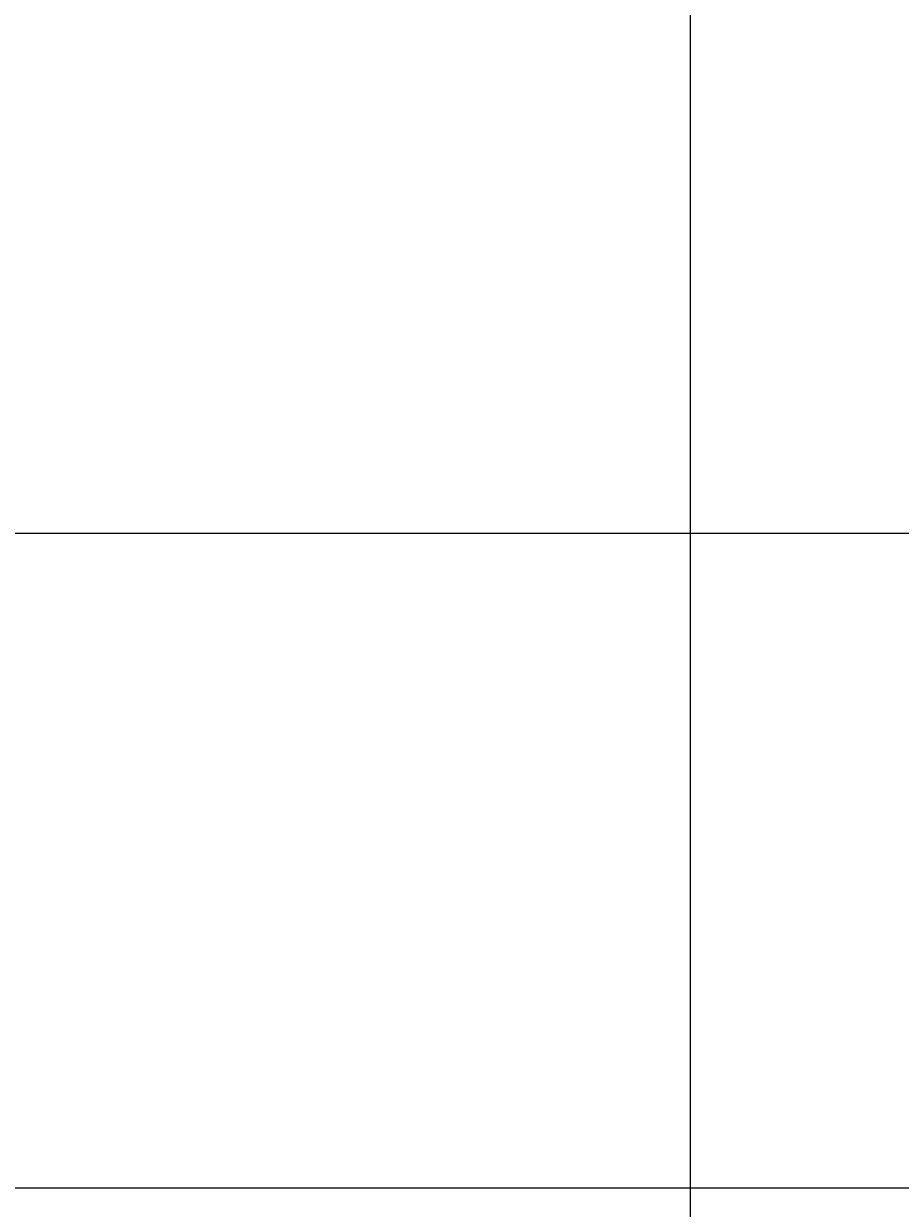
# Model space of a CAD drawing. Units: inches. Extents: x 35362 to 73946, y 43607 to 67532.
# Tile 76 of 134: x 49302 to 50119, y 47689 to 48793. Entities that reach past the tile are written whole.
import ezdxf

# ---------------------------------------------------------------- set-up
doc = ezdxf.new("R2010")
doc.units = ezdxf.units.IN
doc.header["$MEASUREMENT"] = 0
doc.layers.add('A-ANNO-DIMS', color=2, linetype='Continuous', lineweight=18)
doc.styles.get("Standard").update_dxf_attribs({"font": 'arial.ttf'})
doc.dimstyles.get("Standard").update_dxf_attribs({"dimtxt": 0.18, "dimasz": 0.18, "dimexe": 0.18, "dimexo": 0.0625, "dimgap": 0.09, "dimtad": 0, "dimtih": 1, "dimtoh": 1, "dimdec": 4, "dimzin": 0, "dimdsep": 46, "dimtxsty": 'Standard', "dimcen": 0.09, "dimadec": 0, "dimazin": 0, "dimtfac": 1, "dimtdec": 4, "dimtofl": 0, "dimtmove": 0, "dimatfit": 3, "dimfxl": 1, "dimtolj": 1, "dimtzin": 0, "dimarcsym": 0})

# ---------------------------------------------------------------- blocks, each defined once
blk = doc.blocks.new('*D11')
at = {"layer": 'A-ANNO-DIMS', "color": 0, "lineweight": -2, "transparency": 16777216}
for p, q in [((47978.7, 56028.8), (47978.7, 43606.7)), ((53109.8, 56028.8), (53109.8, 43606.7)), ((47978.8, 43606.9), (50543.9, 43606.9)), ((53109.6, 43606.9), (50544.6, 43606.9))]:
    blk.add_line(p, q, dxfattribs=at)
at = {"layer": 'A-ANNO-DIMS', "color": 0, "transparency": 16777216}
for points in [[(47978.8, 43606.9), (47978.8, 43606.8), (47978.7, 43606.9)], [(53109.6, 43606.9), (53109.6, 43606.8), (53109.8, 43606.9)]]:
    blk.add_solid(points, dxfattribs=at)
at = {"layer": 'Defpoints', "color": 0, "transparency": 16777216}
for p in [(47978.7, 56028.8), (53109.8, 56028.8), (53109.8, 43606.9)]:
    blk.add_point(p, dxfattribs=at)
at = {"layer": 'A-ANNO-DIMS', "color": 0, "transparency": 16777216, "insert": (50544.2, 43606.9), "char_height": 0.18, "attachment_point": 5}
blk.add_mtext('\\A1;5131', dxfattribs=at)
blk = doc.blocks.new('*D13')
at = {"layer": 'A-ANNO-DIMS', "color": 0, "lineweight": -2, "transparency": 16777216}
for p, q in [((48373.5, 51694), (48373.5, 43606.7)), ((51029, 51694), (51029, 43606.7)), ((48373.7, 43606.9), (49700.8, 43606.9)), ((51028.9, 43606.9), (49701.7, 43606.9))]:
    blk.add_line(p, q, dxfattribs=at)
at = {"layer": 'A-ANNO-DIMS', "color": 0, "transparency": 16777216}
for points in [[(48373.7, 43606.9), (48373.7, 43606.8), (48373.5, 43606.9)], [(51028.9, 43606.9), (51028.9, 43606.8), (51029, 43606.9)]]:
    blk.add_solid(points, dxfattribs=at)
at = {"layer": 'Defpoints', "color": 0, "transparency": 16777216}
for p in [(48373.5, 51694.1), (51029, 51694.1), (51029, 43606.9)]:
    blk.add_point(p, dxfattribs=at)
at = {"layer": 'A-ANNO-DIMS', "color": 0, "transparency": 16777216, "insert": (49701.3, 43606.9), "char_height": 0.18, "attachment_point": 5}
blk.add_mtext('\\A1;2655.6', dxfattribs=at)
blk = doc.blocks.new('*D17')
at = {"layer": 'A-ANNO-DIMS', "color": 0, "lineweight": -2, "transparency": 16777216}
for p, q in [((49923.3, 61293.2), (49923.3, 43606.7)), ((51913.9, 61293.2), (51913.9, 43606.7)), ((49923.5, 43606.9), (50918.2, 43606.9)), ((51913.8, 43606.9), (50919.1, 43606.9))]:
    blk.add_line(p, q, dxfattribs=at)
at = {"layer": 'A-ANNO-DIMS', "color": 0, "transparency": 16777216}
for points in [[(49923.5, 43606.9), (49923.5, 43606.8), (49923.3, 43606.9)], [(51913.8, 43606.9), (51913.8, 43606.8), (51913.9, 43606.9)]]:
    blk.add_solid(points, dxfattribs=at)
at = {"layer": 'Defpoints', "color": 0, "transparency": 16777216}
for p in [(49923.3, 61293.3), (51913.9, 61293.3), (51913.9, 43606.9)]:
    blk.add_point(p, dxfattribs=at)
at = {"layer": 'A-ANNO-DIMS', "color": 0, "transparency": 16777216, "insert": (50918.6, 43606.9), "char_height": 0.18, "attachment_point": 5}
blk.add_mtext('\\A1;1990.6', dxfattribs=at)
blk = doc.blocks.new('*D67')
at = {"layer": 'A-ANNO-DIMS', "color": 0, "lineweight": -2, "transparency": 16777216}
for p, q in [((56873.5, 53351.5), (35361.8, 53351.5)), ((35361.9, 53351.3), (35361.9, 49400.9)), ((35361.9, 45450.1), (35361.9, 49400.5)), ((53793.6, 45449.9), (35361.8, 45449.9))]:
    blk.add_line(p, q, dxfattribs=at)
at = {"layer": 'A-ANNO-DIMS', "color": 0, "transparency": 16777216}
for points in [[(35361.9, 53351.3), (35362, 53351.3), (35361.9, 53351.5)], [(35361.9, 45450.1), (35362, 45450.1), (35361.9, 45449.9)]]:
    blk.add_solid(points, dxfattribs=at)
at = {"layer": 'Defpoints', "color": 0, "transparency": 16777216}
for p in [(35361.9, 53351.5), (56873.6, 53351.5), (53793.6, 45449.9)]:
    blk.add_point(p, dxfattribs=at)
at = {"layer": 'A-ANNO-DIMS', "color": 0, "transparency": 16777216, "insert": (35361.9, 49400.7), "char_height": 0.18, "attachment_point": 5}
blk.add_mtext('\\A1;7901.6', dxfattribs=at)
blk = doc.blocks.new('*D87')
at = {"layer": 'A-ANNO-DIMS', "color": 0, "lineweight": -2, "transparency": 16777216}
for p, q in [((52362.5, 48318.3), (35361.8, 48318.3)), ((35361.9, 48318.1), (35361.9, 47931.4)), ((35361.9, 47544.3), (35361.9, 47931)), ((52362.5, 47544.1), (35361.8, 47544.1))]:
    blk.add_line(p, q, dxfattribs=at)
at = {"layer": 'A-ANNO-DIMS', "color": 0, "transparency": 16777216}
for points in [[(35361.9, 48318.1), (35362, 48318.1), (35361.9, 48318.3)], [(35361.9, 47544.3), (35362, 47544.3), (35361.9, 47544.1)]]:
    blk.add_solid(points, dxfattribs=at)
at = {"layer": 'Defpoints', "color": 0, "transparency": 16777216}
for p in [(35361.9, 48318.3), (52362.6, 48318.3), (52362.6, 47544.1)]:
    blk.add_point(p, dxfattribs=at)
at = {"layer": 'A-ANNO-DIMS', "color": 0, "transparency": 16777216, "insert": (35361.9, 47931.2), "char_height": 0.18, "attachment_point": 5}
blk.add_mtext('\\A1;774.1', dxfattribs=at)
blk = doc.blocks.new('*D89')
at = {"layer": 'A-ANNO-DIMS', "color": 0, "lineweight": -2, "transparency": 16777216}
for p, q in [((53707.7, 48897.7), (35361.8, 48897.7)), ((35361.9, 48897.6), (35361.9, 48303.2)), ((35361.9, 47708.4), (35361.9, 48302.8)), ((53707.7, 47708.2), (35361.8, 47708.2))]:
    blk.add_line(p, q, dxfattribs=at)
at = {"layer": 'A-ANNO-DIMS', "color": 0, "transparency": 16777216}
for points in [[(35361.9, 48897.6), (35362, 48897.6), (35361.9, 48897.7)], [(35361.9, 47708.4), (35362, 47708.4), (35361.9, 47708.2)]]:
    blk.add_solid(points, dxfattribs=at)
at = {"layer": 'Defpoints', "color": 0, "transparency": 16777216}
for p in [(53707.8, 48897.7), (35361.9, 47708.2), (53707.8, 47708.2)]:
    blk.add_point(p, dxfattribs=at)
at = {"layer": 'A-ANNO-DIMS', "color": 0, "transparency": 16777216, "insert": (35361.9, 48303), "char_height": 0.18, "attachment_point": 5}
blk.add_mtext('\\A1;1189.5', dxfattribs=at)

msp = doc.modelspace()

# ---------------------------------------------------------------- dimensions: what is measured, and where the dimension line sits
at = {"layer": 'A-ANNO-DIMS'}
for base, p1, p2, override, picture, middle in [((51913.931, 43606.859), (49923.307, 61293.286), (51913.931, 61293.286), {"dimdec": 1, "dimlfac": 1, "dimrnd": 0, "dimzin": 0, "dimdsep": 46, "dimlunit": 2}, '*D17', (50918.619, 43606.859)), ((53109.76, 43606.859), (47978.665, 56028.836), (53109.76, 56028.836), {"dimdec": 0, "dimlfac": 1, "dimrnd": 0, "dimzin": 0, "dimdsep": 46, "dimlunit": 2}, '*D11', (50544.212, 43606.859)), ((51029.043, 43606.859), (48373.492, 51694.087), (51029.043, 51694.087), {"dimdec": 1, "dimlfac": 1, "dimrnd": 0, "dimzin": 0, "dimdsep": 46, "dimlunit": 2}, '*D13', (49701.267, 43606.859))]:
    dim = msp.add_linear_dim(base=base, p1=p1, p2=p2, dimstyle='Standard', override=override, dxfattribs=at)
    dim.commit()
    dim.dimension.update_dxf_attribs({"geometry": picture, "text_midpoint": middle})
for base, p1, p2, picture, middle in [((35361.949, 53351.529), (53793.638, 45449.894), (56873.602, 53351.529), '*D67', (35361.949, 49400.712)), ((35361.949, 47708.216), (53707.781, 48897.738), (53707.781, 47708.216), '*D89', (35361.949, 48302.977)), ((35361.949, 48318.269), (52362.557, 47544.134), (52362.557, 48318.269), '*D87', (35361.949, 47931.201))]:
    dim = msp.add_linear_dim(base=base, p1=p1, p2=p2, angle=90, dimstyle='Standard', override={"dimdec": 1, "dimlfac": 1, "dimrnd": 0, "dimzin": 0, "dimdsep": 46, "dimlunit": 2}, dxfattribs=at)
    dim.commit()
    dim.dimension.update_dxf_attribs({"geometry": picture, "text_midpoint": middle})

doc.saveas('drawing.dxf')
